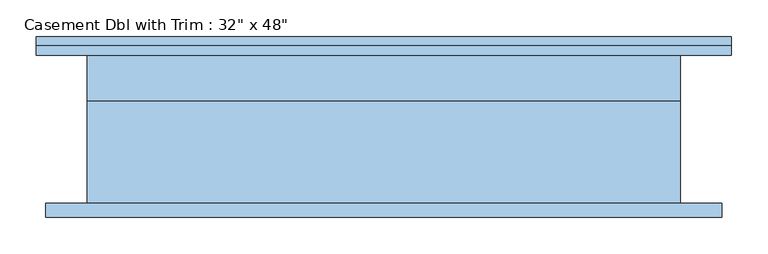
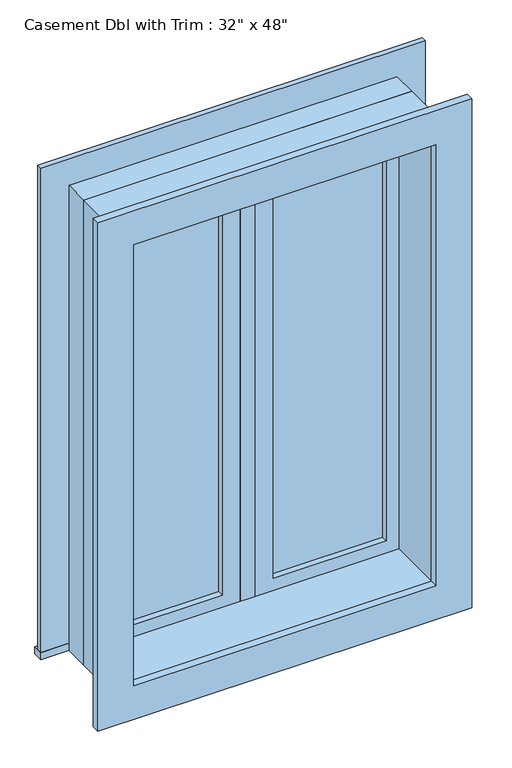
"""IFC4 building model written with IfcOpenShell, lengths in millimetres: window geometry."""

from ifc_helpers import new_model, si_unit, frame, origin, place, context, project, spatial, polyline, outline, extrude, source, transform, mapped, element, save


def window_bb17773d(model_context):
    return source(origin(), model_context, "Body", "SweptSolid", [
        extrude(outline(polyline([(63.5, 85.725), (342.9, 85.725), (342.9, 73.025), (63.5, 73.025), (63.5, 85.725)])), frame((0.0, 0.0, 977.9), z_axis=(0.0, 0.0, 1.0), x_axis=(1.0, 0.0, 0.0)), (0.0, 0.0, 1.0), 1092.2),
        extrude(outline(polyline([(2114.55, 19.05), (933.45, 19.05), (933.45, 387.35), (2114.55, 387.35), (2114.55, 19.05)]), holes=[polyline([(2070.1, 63.5), (2070.1, 342.9), (977.9, 342.9), (977.9, 63.5), (2070.1, 63.5)])]), frame((0.0, 57.15, 0.0), z_axis=(0.0, 1.0, 0.0), x_axis=(0.0, 0.0, 1.0)), (0.0, 0.0, 1.0), 44.45),
        extrude(outline(polyline([(19.05, 57.15), (-19.05, 57.15), (-19.05, 120.65), (19.05, 120.65), (19.05, 57.15)])), frame((0.0, 0.0, 933.45), z_axis=(0.0, 0.0, 1.0), x_axis=(1.0, 0.0, 0.0)), (0.0, 0.0, 1.0), 1181.1),
        extrude(outline(polyline([(-476.25, 146.05), (476.25, 146.05), (476.25, 120.65), (-476.25, 120.65), (-476.25, 146.05)])), frame((0.0, 0.0, 914.4), z_axis=(0.0, 0.0, 1.0), x_axis=(1.0, 0.0, 0.0)), (0.0, 0.0, 1.0), 19.05),
        extrude(outline(polyline([(2114.55, -387.35), (2114.55, 387.35), (933.45, 387.35), (933.45, 476.25), (2203.45, 476.25), (2203.45, -476.25), (933.45, -476.25), (933.45, -387.35), (2114.55, -387.35)])), frame((0.0, 120.65, 0.0), z_axis=(0.0, 1.0, 0.0), x_axis=(0.0, 0.0, 1.0)), (0.0, 0.0, 1.0), 12.7),
        extrude(outline(polyline([(2190.75, 463.55), (2190.75, -463.55), (857.25, -463.55), (857.25, 463.55), (2190.75, 463.55)]), holes=[polyline([(2101.85, 374.65), (946.15, 374.65), (946.15, -374.65), (2101.85, -374.65), (2101.85, 374.65)])]), frame((0.0, -101.6, 0.0), z_axis=(0.0, 1.0, 0.0), x_axis=(0.0, 0.0, 1.0)), (0.0, 0.0, 1.0), 19.05),
        extrude(outline(polyline([(-63.5, 73.025), (-342.9, 73.025), (-342.9, 85.725), (-63.5, 85.725), (-63.5, 73.025)])), frame((0.0, 0.0, 977.9), z_axis=(0.0, 0.0, 1.0), x_axis=(1.0, 0.0, 0.0)), (0.0, 0.0, 1.0), 1092.2),
        extrude(outline(polyline([(2114.55, -387.35), (933.45, -387.35), (933.45, -19.05), (2114.55, -19.05), (2114.55, -387.35)]), holes=[polyline([(2070.1, -342.9), (2070.1, -63.5), (977.9, -63.5), (977.9, -342.9), (2070.1, -342.9)])]), frame((0.0, 57.15, 0.0), z_axis=(0.0, 1.0, 0.0), x_axis=(0.0, 0.0, 1.0)), (0.0, 0.0, 1.0), 44.45),
        extrude(outline(polyline([(2133.6, -406.4), (914.4, -406.4), (914.4, 406.4), (2133.6, 406.4), (2133.6, -406.4)]), holes=[polyline([(2101.85, -374.65), (2101.85, 374.65), (946.15, 374.65), (946.15, -374.65), (2101.85, -374.65)])]), frame((0.0, -82.55, 0.0), z_axis=(0.0, 1.0, 0.0), x_axis=(0.0, 0.0, 1.0)), (0.0, 0.0, 1.0), 139.7),
        extrude(outline(polyline([(2133.6, 406.4), (2133.6, -406.4), (914.4, -406.4), (914.4, 406.4), (2133.6, 406.4)]), holes=[polyline([(2114.55, 387.35), (933.45, 387.35), (933.45, -387.35), (2114.55, -387.35), (2114.55, 387.35)])]), frame((0.0, 57.15, 0.0), z_axis=(0.0, 1.0, 0.0), x_axis=(0.0, 0.0, 1.0)), (0.0, 0.0, 1.0), 63.5),
    ])


if __name__ == "__main__":
    model = new_model("IFC4")
    model_context = context("Model", 3, world=origin())
    ifc_project = project(units=[si_unit("LENGTHUNIT", "METRE", prefix="MILLI")], contexts=[model_context])
    site = spatial("IfcSite", under=ifc_project)
    building = spatial("IfcBuilding", under=site)
    placement = place(None, origin())
    window_shape = window_bb17773d(model_context)
    element("IfcWindow", 1, ObjectType="Casement Dbl with Trim : 32\" x 48\"", at=placement, inside=building, context=model_context, shape_type="MappedRepresentation", body=[
        mapped(window_shape, transform((0.0, 0.0, 0.0), x_axis=(1.0, 0.0, 0.0), y_axis=(0.0, 1.0, 0.0), z_axis=(0.0, 0.0, 1.0))),
    ])
    save(model, "model.ifc")

# Revit data of these elements
# Type "Casement Dbl with Trim : 32\" x 48\""
#   Type Mark = "15"
#   Construction Type Id = "GSP4R"
#   Assembly Code = "B2020100"
#   Analytic Construction = "1/8 in Pilkington single glazing"
#   Visual Light Transmittance = 0.9
#   Solar Heat Gain Coefficient = 0.78
#   Heat Transfer Coefficient (U) = 0.6496 BTU/(h·ft²·°F)
#   Height = 4' - 0"
#   Default Sill Height = 3' - 0"
#   Trim Projection - Ext. = 0' - 0 1/2"
#   Trim Projection - Int. = 0' - 0 3/4"
#   Trim Width - Exterior = 0' - 3 1/2"
#   Trim Width - Interior = 0' - 3 1/2"
#   Width = 2' - 8"
#   Window Inset = 0' - 0 3/4"
#   Define Thermal Properties by = 1
#   Glass Pane Material = Glass
#   Sash Material = Sash
#   Trim Exterior Material = Trim
#   Trim Interior Material = Trim
#   Wall Closure = (empty or 0)
# Element 1 (IfcWindow, "Casement Dbl with Trim : 32\" x 48\"")
#   Materials on its faces: "Sash", "Trim", "Glass"
# Materials
#   "Glass": class "Glass", colour RGB 0 128 192, transparency 0.75, Description = "Soda Lime Glass", Cost = 0
#   "Sash": class "Wood", colour RGB 224 178 126, transparency 0
#   "Trim": class "Wood", colour RGB 224 178 126, transparency 0
